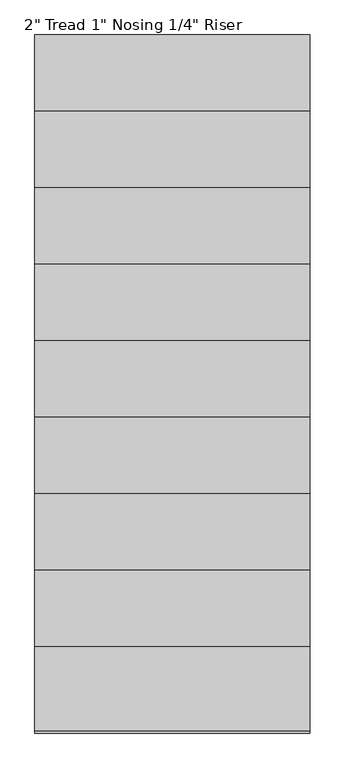
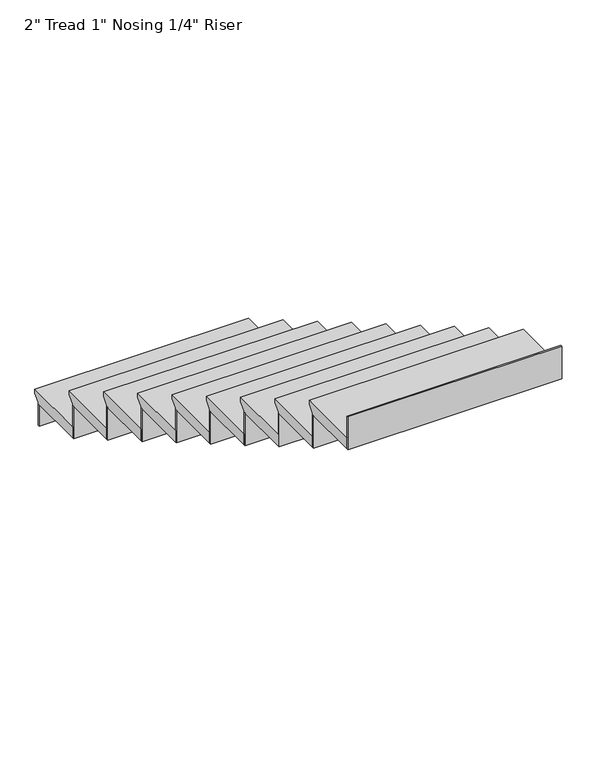
"""IFC4 building model written with IfcOpenShell, lengths in millimetres: stair flight geometry."""

from ifc_helpers import new_model, si_unit, origin, place, context, project, spatial, faceted_brep, source, transform, mapped, element, save


def stair_flight_c4a53ddb(model_context):
    return source(origin(), model_context, "Body", "Brep", [
        faceted_brep([(-4315.1137331, -4241.0593836, 9673.1714861), (-4315.1137331, -4241.0593836, 9692.2214861), (-3400.7137331, -4241.0593836, 9692.2214861), (-3400.7137331, -4241.0593836, 9673.1714861), (-4315.1137331, -4266.4593836, 9647.7714861), (-3400.7137331, -4266.4593836, 9647.7714861), (-4315.1137331, -4520.4593836, 9692.2214861), (-3400.7137331, -4520.4593836, 9692.2214861), (-3400.7137331, -4266.4593836, 9641.4214861), (-3400.7137331, -4520.4593836, 9641.4214861), (-4315.1137331, -4520.4593836, 9641.4214861), (-4315.1137331, -4266.4593836, 9641.4214861)], [[[0, 1, 2, 3]], [[4, 0, 3, 5]], [[2, 1, 6, 7]], [[8, 9, 10, 11]], [[2, 7, 9, 8, 5, 3]], [[8, 11, 4, 5]], [[6, 1, 0, 4, 11, 10]], [[7, 6, 10, 9]]]),
        faceted_brep([(-4315.1137331, -4266.4593836, 9641.4214861), (-4315.1137331, -4266.4593836, 9544.3725604), (-4315.1137331, -4272.8093836, 9544.3725604), (-4315.1137331, -4272.8093836, 9641.4214861), (-3400.7137331, -4266.4593836, 9641.4214861), (-3400.7137331, -4272.8093836, 9641.4214861), (-3400.7137331, -4272.8093836, 9544.3725604), (-3400.7137331, -4266.4593836, 9544.3725604)], [[[0, 1, 2, 3]], [[4, 5, 6, 7]], [[1, 0, 4, 7]], [[2, 1, 7, 6]], [[3, 2, 6, 5]], [[0, 3, 5, 4]]]),
        faceted_brep([(-4315.1137331, -4520.4593836, 9789.2704118), (-4315.1137331, -4520.4593836, 9641.4214861), (-4315.1137331, -4526.8093836, 9641.4214861), (-4315.1137331, -4526.8093836, 9789.2704118), (-3400.7137331, -4520.4593836, 9789.2704118), (-3400.7137331, -4526.8093836, 9789.2704118), (-3400.7137331, -4526.8093836, 9641.4214861), (-3400.7137331, -4520.4593836, 9641.4214861)], [[[0, 1, 2, 3]], [[4, 5, 6, 7]], [[1, 0, 4, 7]], [[2, 1, 7, 6]], [[3, 2, 6, 5]], [[0, 3, 5, 4]]]),
        faceted_brep([(-3400.7137331, -4495.0593836, 9840.0704118), (-4315.1137331, -4495.0593836, 9840.0704118), (-4315.1137331, -4774.4593836, 9840.0704118), (-3400.7137331, -4774.4593836, 9840.0704118), (-3400.7137331, -4520.4593836, 9789.2704118), (-3400.7137331, -4774.4593836, 9789.2704118), (-4315.1137331, -4774.4593836, 9789.2704118), (-4315.1137331, -4520.4593836, 9789.2704118), (-3400.7137331, -4520.4593836, 9795.6204118), (-3400.7137331, -4495.0593836, 9821.0204118), (-4315.1137331, -4520.4593836, 9795.6204118), (-4315.1137331, -4495.0593836, 9821.0204118)], [[[0, 1, 2, 3]], [[4, 5, 6, 7]], [[0, 3, 5, 4, 8, 9]], [[4, 7, 10, 8]], [[2, 1, 11, 10, 7, 6]], [[3, 2, 6, 5]], [[11, 1, 0, 9]], [[10, 11, 9, 8]]]),
        faceted_brep([(-4315.1137331, -4774.4593836, 9937.1193375), (-4315.1137331, -4774.4593836, 9789.2704118), (-4315.1137331, -4780.8093836, 9789.2704118), (-4315.1137331, -4780.8093836, 9937.1193375), (-3400.7137331, -4774.4593836, 9937.1193375), (-3400.7137331, -4780.8093836, 9937.1193375), (-3400.7137331, -4780.8093836, 9789.2704118), (-3400.7137331, -4774.4593836, 9789.2704118)], [[[0, 1, 2, 3]], [[4, 5, 6, 7]], [[1, 0, 4, 7]], [[2, 1, 7, 6]], [[3, 2, 6, 5]], [[0, 3, 5, 4]]]),
        faceted_brep([(-3400.7137331, -4749.0593836, 9987.9193375), (-4315.1137331, -4749.0593836, 9987.9193375), (-4315.1137331, -5028.4593836, 9987.9193375), (-3400.7137331, -5028.4593836, 9987.9193375), (-3400.7137331, -4774.4593836, 9937.1193375), (-3400.7137331, -5028.4593836, 9937.1193375), (-4315.1137331, -5028.4593836, 9937.1193375), (-4315.1137331, -4774.4593836, 9937.1193375), (-3400.7137331, -4774.4593836, 9943.4693375), (-3400.7137331, -4749.0593836, 9968.8693375), (-4315.1137331, -4774.4593836, 9943.4693375), (-4315.1137331, -4749.0593836, 9968.8693375)], [[[0, 1, 2, 3]], [[4, 5, 6, 7]], [[0, 3, 5, 4, 8, 9]], [[4, 7, 10, 8]], [[2, 1, 11, 10, 7, 6]], [[3, 2, 6, 5]], [[11, 1, 0, 9]], [[10, 11, 9, 8]]]),
        faceted_brep([(-4315.1137331, -5028.4593836, 10084.9682632), (-4315.1137331, -5028.4593836, 9937.1193375), (-4315.1137331, -5034.8093836, 9937.1193375), (-4315.1137331, -5034.8093836, 10084.9682632), (-3400.7137331, -5028.4593836, 10084.9682632), (-3400.7137331, -5034.8093836, 10084.9682632), (-3400.7137331, -5034.8093836, 9937.1193375), (-3400.7137331, -5028.4593836, 9937.1193375)], [[[0, 1, 2, 3]], [[4, 5, 6, 7]], [[1, 0, 4, 7]], [[2, 1, 7, 6]], [[3, 2, 6, 5]], [[0, 3, 5, 4]]]),
        faceted_brep([(-3400.7137331, -5003.0593836, 10135.7682632), (-4315.1137331, -5003.0593836, 10135.7682632), (-4315.1137331, -5282.4593836, 10135.7682632), (-3400.7137331, -5282.4593836, 10135.7682632), (-3400.7137331, -5028.4593836, 10084.9682632), (-3400.7137331, -5282.4593836, 10084.9682632), (-4315.1137331, -5282.4593836, 10084.9682632), (-4315.1137331, -5028.4593836, 10084.9682632), (-3400.7137331, -5028.4593836, 10091.3182632), (-3400.7137331, -5003.0593836, 10116.7182632), (-4315.1137331, -5028.4593836, 10091.3182632), (-4315.1137331, -5003.0593836, 10116.7182632)], [[[0, 1, 2, 3]], [[4, 5, 6, 7]], [[0, 3, 5, 4, 8, 9]], [[4, 7, 10, 8]], [[2, 1, 11, 10, 7, 6]], [[3, 2, 6, 5]], [[11, 1, 0, 9]], [[10, 11, 9, 8]]]),
        faceted_brep([(-4315.1137331, -5282.4593836, 10232.8171889), (-4315.1137331, -5282.4593836, 10084.9682632), (-4315.1137331, -5288.8093836, 10084.9682632), (-4315.1137331, -5288.8093836, 10232.8171889), (-3400.7137331, -5282.4593836, 10232.8171889), (-3400.7137331, -5288.8093836, 10232.8171889), (-3400.7137331, -5288.8093836, 10084.9682632), (-3400.7137331, -5282.4593836, 10084.9682632)], [[[0, 1, 2, 3]], [[4, 5, 6, 7]], [[1, 0, 4, 7]], [[2, 1, 7, 6]], [[3, 2, 6, 5]], [[0, 3, 5, 4]]]),
        faceted_brep([(-3400.7137331, -5257.0593836, 10283.6171889), (-4315.1137331, -5257.0593836, 10283.6171889), (-4315.1137331, -5536.4593836, 10283.6171889), (-3400.7137331, -5536.4593836, 10283.6171889), (-3400.7137331, -5282.4593836, 10232.8171889), (-3400.7137331, -5536.4593836, 10232.8171889), (-4315.1137331, -5536.4593836, 10232.8171889), (-4315.1137331, -5282.4593836, 10232.8171889), (-3400.7137331, -5282.4593836, 10239.1671889), (-3400.7137331, -5257.0593836, 10264.5671889), (-4315.1137331, -5282.4593836, 10239.1671889), (-4315.1137331, -5257.0593836, 10264.5671889)], [[[0, 1, 2, 3]], [[4, 5, 6, 7]], [[0, 3, 5, 4, 8, 9]], [[4, 7, 10, 8]], [[2, 1, 11, 10, 7, 6]], [[3, 2, 6, 5]], [[11, 1, 0, 9]], [[10, 11, 9, 8]]]),
        faceted_brep([(-4315.1137331, -5536.4593836, 10380.6661146), (-4315.1137331, -5536.4593836, 10232.8171889), (-4315.1137331, -5542.8093836, 10232.8171889), (-4315.1137331, -5542.8093836, 10380.6661146), (-3400.7137331, -5536.4593836, 10380.6661146), (-3400.7137331, -5542.8093836, 10380.6661146), (-3400.7137331, -5542.8093836, 10232.8171889), (-3400.7137331, -5536.4593836, 10232.8171889)], [[[0, 1, 2, 3]], [[4, 5, 6, 7]], [[1, 0, 4, 7]], [[2, 1, 7, 6]], [[3, 2, 6, 5]], [[0, 3, 5, 4]]]),
        faceted_brep([(-3400.7137331, -5511.0593836, 10431.4661146), (-4315.1137331, -5511.0593836, 10431.4661146), (-4315.1137331, -5790.4593836, 10431.4661146), (-3400.7137331, -5790.4593836, 10431.4661146), (-3400.7137331, -5536.4593836, 10380.6661146), (-3400.7137331, -5790.4593836, 10380.6661146), (-4315.1137331, -5790.4593836, 10380.6661146), (-4315.1137331, -5536.4593836, 10380.6661146), (-3400.7137331, -5536.4593836, 10387.0161146), (-3400.7137331, -5511.0593836, 10412.4161146), (-4315.1137331, -5536.4593836, 10387.0161146), (-4315.1137331, -5511.0593836, 10412.4161146)], [[[0, 1, 2, 3]], [[4, 5, 6, 7]], [[0, 3, 5, 4, 8, 9]], [[4, 7, 10, 8]], [[2, 1, 11, 10, 7, 6]], [[3, 2, 6, 5]], [[11, 1, 0, 9]], [[10, 11, 9, 8]]]),
        faceted_brep([(-4315.1137331, -5790.4593836, 10528.5150403), (-4315.1137331, -5790.4593836, 10380.6661146), (-4315.1137331, -5796.8093836, 10380.6661146), (-4315.1137331, -5796.8093836, 10528.5150403), (-3400.7137331, -5790.4593836, 10528.5150403), (-3400.7137331, -5796.8093836, 10528.5150403), (-3400.7137331, -5796.8093836, 10380.6661146), (-3400.7137331, -5790.4593836, 10380.6661146)], [[[0, 1, 2, 3]], [[4, 5, 6, 7]], [[1, 0, 4, 7]], [[2, 1, 7, 6]], [[3, 2, 6, 5]], [[0, 3, 5, 4]]]),
        faceted_brep([(-3400.7137331, -5765.0593836, 10579.3150403), (-4315.1137331, -5765.0593836, 10579.3150403), (-4315.1137331, -6044.4593836, 10579.3150403), (-3400.7137331, -6044.4593836, 10579.3150403), (-3400.7137331, -5790.4593836, 10528.5150403), (-3400.7137331, -6044.4593836, 10528.5150403), (-4315.1137331, -6044.4593836, 10528.5150403), (-4315.1137331, -5790.4593836, 10528.5150403), (-3400.7137331, -5790.4593836, 10534.8650403), (-3400.7137331, -5765.0593836, 10560.2650403), (-4315.1137331, -5790.4593836, 10534.8650403), (-4315.1137331, -5765.0593836, 10560.2650403)], [[[0, 1, 2, 3]], [[4, 5, 6, 7]], [[0, 3, 5, 4, 8, 9]], [[4, 7, 10, 8]], [[2, 1, 11, 10, 7, 6]], [[3, 2, 6, 5]], [[11, 1, 0, 9]], [[10, 11, 9, 8]]]),
        faceted_brep([(-4315.1137331, -6044.4593836, 10676.363966), (-4315.1137331, -6044.4593836, 10528.5150403), (-4315.1137331, -6050.8093836, 10528.5150403), (-4315.1137331, -6050.8093836, 10676.363966), (-3400.7137331, -6044.4593836, 10676.363966), (-3400.7137331, -6050.8093836, 10676.363966), (-3400.7137331, -6050.8093836, 10528.5150403), (-3400.7137331, -6044.4593836, 10528.5150403)], [[[0, 1, 2, 3]], [[4, 5, 6, 7]], [[1, 0, 4, 7]], [[2, 1, 7, 6]], [[3, 2, 6, 5]], [[0, 3, 5, 4]]]),
        faceted_brep([(-3400.7137331, -6019.0593836, 10727.163966), (-4315.1137331, -6019.0593836, 10727.163966), (-4315.1137331, -6298.4593836, 10727.163966), (-3400.7137331, -6298.4593836, 10727.163966), (-3400.7137331, -6044.4593836, 10676.363966), (-3400.7137331, -6298.4593836, 10676.363966), (-4315.1137331, -6298.4593836, 10676.363966), (-4315.1137331, -6044.4593836, 10676.363966), (-3400.7137331, -6044.4593836, 10682.713966), (-3400.7137331, -6019.0593836, 10708.113966), (-4315.1137331, -6044.4593836, 10682.713966), (-4315.1137331, -6019.0593836, 10708.113966)], [[[0, 1, 2, 3]], [[4, 5, 6, 7]], [[0, 3, 5, 4, 8, 9]], [[4, 7, 10, 8]], [[2, 1, 11, 10, 7, 6]], [[3, 2, 6, 5]], [[11, 1, 0, 9]], [[10, 11, 9, 8]]]),
        faceted_brep([(-4315.1137331, -6552.4593836, 10972.0618174), (-4315.1137331, -6552.4593836, 10824.2128917), (-4315.1137331, -6558.8093836, 10824.2128917), (-4315.1137331, -6558.8093836, 10972.0618174), (-3400.7137331, -6552.4593836, 10972.0618174), (-3400.7137331, -6558.8093836, 10972.0618174), (-3400.7137331, -6558.8093836, 10824.2128917), (-3400.7137331, -6552.4593836, 10824.2128917)], [[[0, 1, 2, 3]], [[4, 5, 6, 7]], [[1, 0, 4, 7]], [[2, 1, 7, 6]], [[3, 2, 6, 5]], [[0, 3, 5, 4]]]),
        faceted_brep([(-4315.1137331, -6298.4593836, 10824.2128917), (-4315.1137331, -6298.4593836, 10676.363966), (-4315.1137331, -6304.8093836, 10676.363966), (-4315.1137331, -6304.8093836, 10824.2128917), (-3400.7137331, -6298.4593836, 10824.2128917), (-3400.7137331, -6304.8093836, 10824.2128917), (-3400.7137331, -6304.8093836, 10676.363966), (-3400.7137331, -6298.4593836, 10676.363966)], [[[0, 1, 2, 3]], [[4, 5, 6, 7]], [[1, 0, 4, 7]], [[2, 1, 7, 6]], [[3, 2, 6, 5]], [[0, 3, 5, 4]]]),
        faceted_brep([(-3400.7137331, -6552.4593836, 10875.0128917), (-3400.7137331, -6527.0593836, 10875.0128917), (-3400.7137331, -6273.0593836, 10875.0128917), (-4315.1137331, -6273.0593836, 10875.0128917), (-4315.1137331, -6552.4593836, 10875.0128917), (-3400.7137331, -6527.0593836, 10824.2128917), (-3400.7137331, -6552.4593836, 10824.2128917), (-4315.1137331, -6552.4593836, 10824.2128917), (-4315.1137331, -6298.4593836, 10824.2128917), (-3400.7137331, -6298.4593836, 10824.2128917), (-3400.7137331, -6298.4593836, 10830.5628917), (-3400.7137331, -6273.0593836, 10855.9628917), (-4315.1137331, -6298.4593836, 10830.5628917), (-4315.1137331, -6273.0593836, 10855.9628917)], [[[0, 1, 2, 3, 4]], [[5, 6, 7, 8, 9]], [[1, 0, 6, 5]], [[2, 1, 5, 9, 10, 11]], [[9, 8, 12, 10]], [[4, 3, 13, 12, 8, 7]], [[0, 4, 7, 6]], [[13, 3, 2, 11]], [[12, 13, 11, 10]]]),
    ])


if __name__ == "__main__":
    model = new_model("IFC4")
    model_context = context("Model", 3, world=origin())
    ifc_project = project(units=[si_unit("LENGTHUNIT", "METRE", prefix="MILLI")], contexts=[model_context])
    site = spatial("IfcSite", under=ifc_project)
    building = spatial("IfcBuilding", under=site)
    placement = place(None, origin())
    stair_flight_shape = stair_flight_c4a53ddb(model_context)
    element("IfcStairFlight", 1, ObjectType="2\" Tread 1\" Nosing 1/4\" Riser", at=placement, inside=building, context=model_context, shape_type="MappedRepresentation", body=[
        mapped(stair_flight_shape, transform((0.0, 0.0, 0.0), x_axis=(1.0, 0.0, 0.0), y_axis=(0.0, 1.0, 0.0), z_axis=(0.0, 0.0, 1.0))),
    ])
    save(model, "model.ifc")
